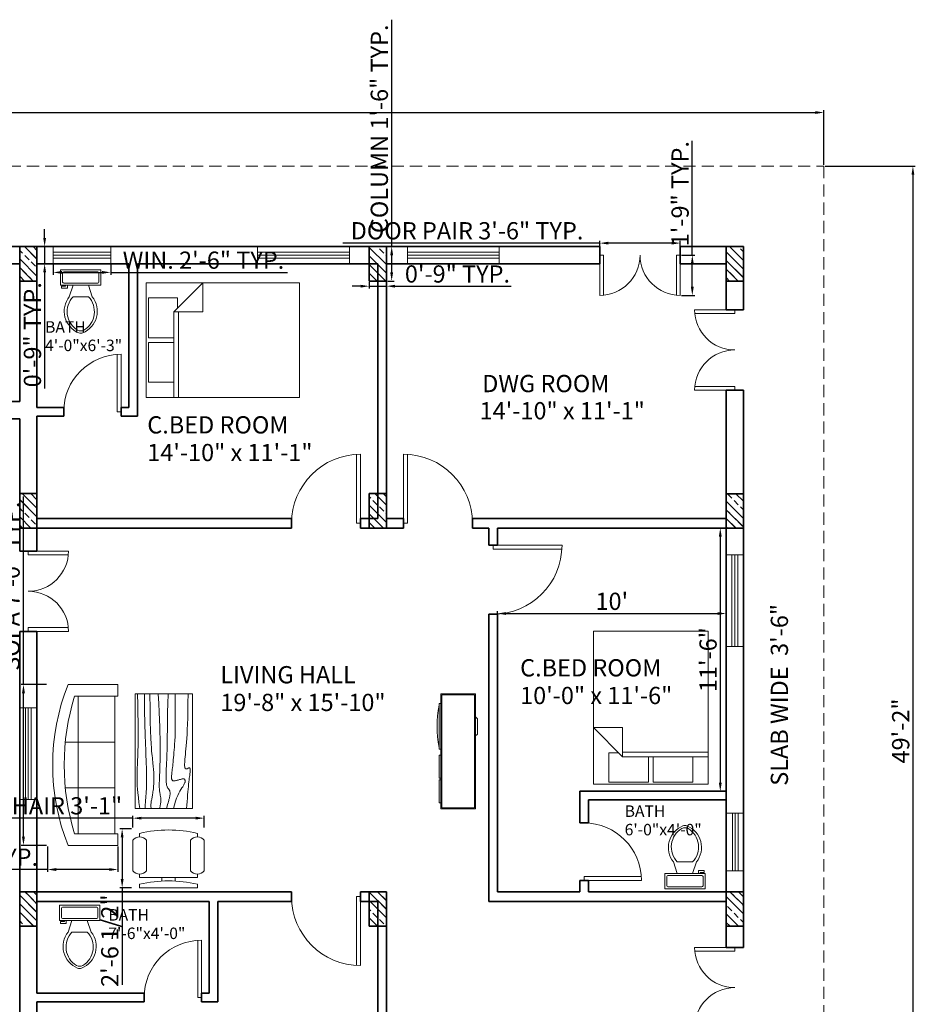
# Model space of a CAD drawing. Units: inches. Extents: x 2081 to 4786, y 1256 to 3802.
# Tile 7 of 7: x 2685 to 3153, y 1585 to 2100. Entities that reach past the tile are written whole.
import ezdxf

# ---------------------------------------------------------------- set-up
doc = ezdxf.new("R2010")
doc.units = ezdxf.units.IN
doc.linetypes.add('HIDDEN', pattern=[9.525, 6.35, -3.175])
for name, color, linetype, lineweight in [('A-ANNO-DIMS', 18, 'Continuous', 18), ('A-ANNO-TEXT', 18, 'Continuous', 18), ('A-AREA-IDEN', 18, 'Continuous', 18), ('A-COLS', 1, 'Continuous', 35), ('A-DOOR', 5, 'Continuous', 18), ('A-FLOR-FIXT', 18, 'Continuous', 18), ('A-FLOR-OVHD', 18, 'HIDDEN', 18), ('A-FURN', 5, 'Continuous', 18), ('A-GLAZ', 11, 'Continuous', 18), ('A-WALL', 7, 'Continuous', 35)]:
    doc.layers.add(name, color=color, linetype=linetype, lineweight=lineweight)
doc.styles.get("Standard").update_dxf_attribs({"font": 'arial.ttf'})
doc.dimstyles.new('ISO-25', dxfattribs={"dimtxt": 9, "dimasz": 4.5, "dimexe": 1.25, "dimexo": 0.625, "dimtad": 1, "dimdec": 0, "dimlunit": 3, "dimtxsty": 'Standard', "dimcen": 2.5, "dimadec": 0, "dimazin": 0, "dimtfac": 1, "dimtdec": 0, "dimtmove": 0, "dimatfit": 3, "dimfxl": 1, "dimarcsym": 0})
pattern_1 = [(135, (1916.44, -3174.735), (-13.47038, -13.47038), []), (135, (1916.44, -3170.245), (-13.47038, -13.47038), []), (135, (1916.44, -3165.755), (-13.47038, -13.47038), []), (135, (1916.44, -3161.265), (-13.47038, -13.47038), [])]

# ---------------------------------------------------------------- blocks, each defined once
blk = doc.blocks.new('Bed - Queen')
for p, q in [((0, -80.00003), (0, 0)), ((0, 0), (59.99999, 0)), ((59.99999, 0), (59.99999, -80.00003)), ((7.99999, -1.2), (28.79998, -1.2)), ((7.99999, -14.4), (7.99999, -1.2)), ((28.79998, -1.2), (28.79998, -14.4)), ((31.19999, -1.2), (51.99999, -1.2)), ((31.19999, -14.4), (31.19999, -1.2)), ((51.99999, -1.2), (51.99999, -16.4)), ((0, -14.4), (44.8, -14.4)), ((59.99999, -29.6), (44.8, -14.4)), ((44.8, -14.4), (44.8, -29.6)), ((44.8, -16.8), (0, -16.8)), ((51.99999, -16.4), (46.79936, -16.4)), ((44.8, -29.6), (59.99999, -29.6)), ((59.99999, -80.00003), (0, -80.00003))]:
    blk.add_line(p, q)
blk = doc.blocks.new('Sofa - Roundback 7 ft.')
for p, q in [((-12.00002, -32.4421), (-12.00003, -6.5971)), ((11.99997, -32.4421), (11.99998, -6.5971)), ((-36.000027, -34), (-36.000027, -11.4696)), ((-35.999844, -13.3819), (35.9998, -13.3819)), ((35.99998, -34), (35.99998, -11.4696)), ((-36.000027, -32.4421), (35.99998, -32.4421))]:
    blk.add_line(p, q)
for points in [[(-36.000027, -34), (-42.000027, -34), (-42.000027, -8)], [(41.99998, -8), (41.99998, -34), (35.99998, -34)]]:
    blk.add_lwpolyline(points)
for centre, radius, start, end in [((0, -114.25), 114.25, 68.43141, 111.5686), ((-0.00001, -127.1968), 121.1968, 72.72033, 107.2797)]:
    blk.add_arc(centre, radius, start, end)
blk = doc.blocks.new('Table - Rectangular Woodgrain 60 x 30 in.')
for p, q in [((0, 0), (0, -30)), ((60, 0), (0, 0)), ((60, -30), (60, 0)), ((0, -30), (60, -30))]:
    blk.add_line(p, q)
for points in [[(0, -2.4), (4.8155, -2.418), (9.0302, -2.4688), (12.709, -2.5477), (15.9167, -2.65), (18.7181, -2.7711), (21.1781, -2.9063), (23.3616, -3.0508), (25.3333, -3.2), (27.1477, -3.3495), (28.8172, -3.4958), (30.3437, -3.636), (31.7291, -3.7667), (32.9756, -3.8849), (34.0849, -3.9875), (35.059, -4.0714), (35.9, -4.1334), (36.6114, -4.1711), (37.2041, -4.1854), (37.6906, -4.1779), (38.0833, -4.15), (38.3948, -4.1034), (38.6375, -4.0396), (38.8239, -3.9602), (38.9666, -3.8667), (39.0764, -3.7608), (39.1573, -3.6448), (39.2116, -3.521), (39.2416, -3.3917), (39.2498, -3.2593), (39.2385, -3.1261), (39.21, -2.9944), (39.1666, -2.8667), (39.111, -2.7447), (39.0468, -2.6281), (38.978, -2.5163), (38.9083, -2.4083), (38.8418, -2.3035), (38.7823, -2.201), (38.7337, -2.1001), (38.7, -2), (38.6844, -1.9003), (38.6875, -1.8021), (38.7094, -1.707), (38.75, -1.6167), (38.8094, -1.5326), (38.8875, -1.4563), (38.9844, -1.3893), (39.1, -1.3333), (39.2351, -1.2896), (39.3937, -1.2583), (39.5804, -1.2396), (39.8, -1.2333), (40.057, -1.2396), (40.3562, -1.2583), (40.7023, -1.2896), (41.1, -1.3333), (41.5547, -1.3895), (42.0755, -1.4573), (42.6721, -1.5361), (43.3542, -1.625), (44.1316, -1.7233), (45.014, -1.8302), (46.0114, -1.9449), (47.1333, -2.0667), (48.3862, -2.1947), (49.7625, -2.3281), (51.2513, -2.4663), (52.8416, -2.6083), (54.5226, -2.7535), (56.2833, -2.9011), (58.1127, -3.0501), (60, -3.2)], [(0, -9.2), (6.5759, -9.0858), (11.9385, -9.0365), (16.2527, -9.0418), (19.6833, -9.0917), (22.3952, -9.1759), (24.5531, -9.2844), (26.322, -9.4069), (27.8666, -9.5333), (29.3241, -9.6553), (30.7203, -9.7719), (32.0532, -9.8837), (33.3208, -9.9917), (34.5213, -10.0965), (35.6526, -10.199), (36.7128, -10.2999), (37.7, -10.4), (38.6129, -10.4996), (39.4531, -10.5969), (40.223, -10.6895), (40.925, -10.775), (41.5613, -10.8512), (42.1344, -10.9156), (42.6465, -10.966), (43.1, -11), (43.4976, -11.0158), (43.8437, -11.0136), (44.143, -10.9942), (44.4, -10.9583), (44.6195, -10.9069), (44.8062, -10.8406), (44.9648, -10.7603), (45.1, -10.6667), (45.2155, -10.5598), (45.3114, -10.4365), (45.3871, -10.2929), (45.4416, -10.125), (45.4743, -9.929), (45.4844, -9.7011), (45.4709, -9.4371), (45.4333, -9.1333), (45.3716, -8.7883), (45.2896, -8.4104), (45.1919, -8.0107), (45.0833, -7.6), (44.9685, -7.1893), (44.8521, -6.7896), (44.7388, -6.4117), (44.6333, -6.0667), (44.54, -5.7628), (44.4614, -5.4979), (44.4001, -5.2675), (44.3583, -5.0667), (44.3384, -4.8909), (44.3427, -4.7354), (44.3736, -4.5956), (44.4333, -4.4667), (44.5236, -4.3453), (44.6427, -4.2333), (44.7884, -4.1339), (44.9583, -4.05), (45.1501, -3.9849), (45.3614, -3.9417), (45.59, -3.9234), (45.8333, -3.9333), (46.0915, -3.9749), (46.3734, -4.0531), (46.6906, -4.1736), (47.0542, -4.3417), (47.4756, -4.5629), (47.9661, -4.8427), (48.5372, -5.1866), (49.2, -5.6), (49.9676, -6.0844), (50.8594, -6.625), (51.8965, -7.2031), (53.1, -7.8), (54.491, -8.3969), (56.0906, -8.975), (57.9199, -9.5156), (60, -10)], [(0, -12.8), (5.1847, -12.9322), (9.6213, -13.0323), (13.3963, -13.1059), (16.5958, -13.1583), (19.3063, -13.1952), (21.614, -13.2219), (23.6054, -13.2439), (25.3666, -13.2667), (26.9728, -13.2947), (28.4531, -13.3281), (29.8256, -13.3663), (31.1083, -13.4083), (32.3191, -13.4535), (33.476, -13.501), (34.597, -13.5501), (35.7, -13.6), (36.7984, -13.6497), (37.8875, -13.6979), (38.9578, -13.743), (40, -13.7833), (41.0047, -13.8174), (41.9625, -13.8438), (42.864, -13.8607), (43.7, -13.8667), (44.4631, -13.8604), (45.1552, -13.8417), (45.7801, -13.8104), (46.3416, -13.7667), (46.8439, -13.7104), (47.2906, -13.6417), (47.6858, -13.5604), (48.0333, -13.4667), (48.3375, -13.3608), (48.6042, -13.2448), (48.8396, -13.121), (49.05, -12.9917), (49.2417, -12.8593), (49.4208, -12.7261), (49.5937, -12.5944), (49.7667, -12.4667), (49.9452, -12.3451), (50.1323, -12.2313), (50.3303, -12.1268), (50.5416, -12.0333), (50.7686, -11.9524), (51.0135, -11.8854), (51.2788, -11.8341), (51.5666, -11.8), (51.8785, -11.7843), (52.2116, -11.7865), (52.562, -11.8059), (52.926, -11.8417), (53.2998, -11.8931), (53.6795, -11.9594), (54.0614, -12.0397), (54.4416, -12.1333), (54.8223, -12.2401), (55.2293, -12.3625), (55.6942, -12.5037), (56.2489, -12.6667), (56.9251, -12.8547), (57.7545, -13.0708), (58.7689, -13.3182), (60, -13.6)], [(0, -18), (5.124, -17.7273), (9.6609, -17.5057), (13.6705, -17.3303), (17.2125, -17.1958), (20.3467, -17.0973), (23.1328, -17.0297), (25.6307, -16.9878), (27.9, -16.9667), (29.9928, -16.9617), (31.9302, -16.9703), (33.7254, -16.9907), (35.3917, -17.0208), (36.9423, -17.0588), (38.3906, -17.1026), (39.7499, -17.1503), (41.0333, -17.2), (42.2519, -17.2496), (43.4073, -17.2969), (44.4986, -17.3395), (45.525, -17.375), (46.4858, -17.4012), (47.3802, -17.4156), (48.2074, -17.416), (48.9667, -17.4), (49.6583, -17.3662), (50.2872, -17.3167), (50.8595, -17.2547), (51.3812, -17.1833), (51.8584, -17.1057), (52.2971, -17.025), (52.7034, -16.9443), (53.0833, -16.8667), (53.443, -16.7951), (53.789, -16.7313), (54.128, -16.6768), (54.4666, -16.6334), (54.8115, -16.6024), (55.1693, -16.5854), (55.5465, -16.5841), (55.95, -16.6), (56.3828, -16.6337), (56.8346, -16.6823), (57.2915, -16.7418), (57.7396, -16.8084), (58.165, -16.878), (58.5539, -16.9469), (58.8924, -17.0111), (59.1666, -17.0667), (59.3679, -17.1107), (59.5078, -17.1438), (59.6032, -17.1675), (59.6708, -17.1833), (59.7275, -17.193), (59.7901, -17.1979), (59.8753, -17.1998), (60, -17.2)], [(0, -22.4), (8.0098, -22.2501), (14.4094, -22.1011), (19.4168, -21.9535), (23.25, -21.8083), (26.1269, -21.6663), (28.2656, -21.5281), (29.884, -21.3947), (31.2, -21.2667), (32.3967, -21.1448), (33.5172, -21.0292), (34.5697, -20.9198), (35.5625, -20.8167), (36.5037, -20.7198), (37.4015, -20.6292), (38.2642, -20.5448), (39.1, -20.4667), (39.9164, -20.3951), (40.7187, -20.3313), (41.5117, -20.2768), (42.3, -20.2333), (43.0883, -20.2024), (43.8812, -20.1854), (44.6836, -20.1841), (45.5, -20.2), (46.3328, -20.234), (47.1747, -20.2844), (48.0163, -20.3488), (48.8479, -20.425), (49.66, -20.5106), (50.4429, -20.6031), (51.1872, -20.7004), (51.8833, -20.8), (52.5246, -20.8999), (53.1166, -20.9995), (53.6681, -21.0983), (54.1875, -21.1958), (54.6834, -21.2919), (55.1646, -21.3859), (55.6394, -21.4777), (56.1167, -21.5667), (56.6028, -21.6515), (57.0961, -21.7266), (57.5929, -21.7852), (58.0896, -21.8208), (58.5823, -21.8268), (59.0674, -21.7964), (59.5412, -21.723), (60, -21.6)], [(0, -25.2), (8.6355, -25.0504), (15.7026, -24.9031), (21.4049, -24.7606), (25.9458, -24.625), (29.529, -24.4988), (32.3578, -24.3844), (34.6359, -24.284), (36.5667, -24.2), (38.3213, -24.1341), (39.9417, -24.0854), (41.437, -24.0523), (42.8167, -24.0333), (44.0901, -24.0268), (45.2667, -24.0313), (46.3557, -24.0451), (47.3667, -24.0667), (48.309, -24.0947), (49.1928, -24.1287), (50.0284, -24.168), (50.826, -24.2125), (51.5959, -24.2617), (52.3483, -24.3151), (53.0935, -24.3725), (53.8417, -24.4334), (54.6009, -24.497), (55.3699, -24.561), (56.1454, -24.6226), (56.9239, -24.6792), (57.7021, -24.7279), (58.4764, -24.7662), (59.2435, -24.7911), (60, -24.8)], [(0, -28.8), (5.6867, -28.6681), (10.45, -28.5698), (14.407, -28.5012), (17.675, -28.4584), (20.3711, -28.4374), (22.6125, -28.4344), (24.5164, -28.4455), (26.2, -28.4667), (27.762, -28.4947), (29.2276, -28.5281), (30.6033, -28.5663), (31.8958, -28.6084), (33.1118, -28.6535), (34.2578, -28.7011), (35.3405, -28.7501), (36.3666, -28.8), (37.3443, -28.8497), (38.288, -28.8974), (39.2137, -28.9412), (40.1375, -28.9792), (41.0753, -29.0093), (42.0432, -29.0297), (43.0572, -29.0384), (44.1333, -29.0333), (45.2936, -29.0114), (46.5843, -28.9641), (48.0579, -28.8816), (49.7666, -28.7542), (51.7629, -28.5721), (54.0989, -28.3255), (56.8272, -28.0048), (60, -27.6)]]:
    blk.add_lwpolyline(points)
blk = doc.blocks.new('Entertainment Center')
for p, q in [((-4, 0), (-5, -1)), ((4, 0), (-4, 0)), ((5, -1), (4, 0)), ((-17, -19), (-17, -1)), ((-17, -1), (43, -1)), ((-16.5, -18.5), (-16.5, -1.5)), ((-16.5, -1.5), (42.5, -1.5)), ((42.5, -1.5), (42.5, -18.5)), ((43, -1), (43, -19)), ((43, -19), (-17, -19)), ((42.5, -18.5), (-16.5, -18.5)), ((-12, -20), (-12, -19)), ((12, -20), (-12, -20)), ((12, -19), (12, -20)), ((15, -20), (15, -19)), ((27, -20), (15, -20)), ((27, -19), (27, -20)), ((28, -20), (28, -19)), ((40, -20), (28, -20)), ((40, -19), (40, -20))]:
    blk.add_line(p, q)
blk.add_arc((0, 40), 61, 259.6111, 280.3889)
blk = doc.blocks.new('Chair - Desk')
for p, q in [((-8.5, 0), (-8.5, -1)), ((-8.5, 0), (8.5, 0)), ((8.5, 0), (8.5, -1)), ((-2, -3), (-2, -1.9355)), ((2, -1.9576), (2, -3)), ((-10.5, -5), (-10.5, -14)), ((-8.5, -3), (-8.5, -4)), ((-8.5, -3), (8.5, -3)), ((-6.5, -14), (-6.5, -5)), ((6.5, -5), (6.5, -14)), ((8.5, -3), (8.5, -4)), ((10.5, -14), (10.5, -5)), ((-8.5, -15), (-8.5, -16)), ((8.5, -15), (8.5, -16))]:
    blk.add_line(p, q)
for centre, radius, start, end in [((0, 34.625), 36.625, 256.5803, 283.4197), ((-8.5, -6.5), 2.5, 36.8699, 143.1301), ((8.5, -6.5), 2.5, 36.8699, 143.1301), ((-8.5, -12.5), 2.5, 216.8699, 323.1301), ((8.5, -12.5), 2.5, 216.8699, 323.1301), ((0, 19.625), 36.625, 256.5803, 283.4197)]:
    blk.add_arc(centre, radius, start, end)
blk = doc.blocks.new('Toilet - top')
for p, q in [((9.5, -6), (9.5, -2)), ((-10, -8.5), (-8, -8.5)), ((-10, -9.5), (-10, -8.5)), ((-7, -9.5), (-10, -9.5)), ((-8, -8.5), (-8, -8)), ((-7, -8), (-7, -9.5)), ((-4, -8), (-6, -14)), ((4, -8), (6, -14)), ((4, -14), (-4, -14))]:
    blk.add_line(p, q)
blk.add_lwpolyline([(10.5, -8), (10.5, 0), (-10.5, 0), (-10.5, -8)], close=True)
for points in [[(-9.5, -2), (-9.5, -6)], [(8.5, -1), (-8.5, -1)], [(-8.5, -7), (8.5, -7)]]:
    blk.add_lwpolyline(points)
for centre, radius, start, end in [((-8.62, -1.88), 0.884, 81.8699, 188.1301), ((8.62, -1.88), 0.884, 351.8699, 98.1301), ((-8.62, -6.12), 0.884, 171.8699, 278.1301), ((8.62, -6.12), 0.884, 261.8699, 8.1301), ((3.52, -21.58), 12.17, 141.4691, 247.9714), ((4.2, -21.82), 11.33, 136.3677, 238.9468), ((-3.52, -21.58), 12.17, 292.0284, 38.5307), ((-4.2, -21.82), 11.33, 301.053, 43.6321), ((0, -27.88), 4, 245.7318, 294.2682), ((0, -29), 4, 254.8605, 285.1395)]:
    blk.add_arc(centre, radius, start, end)
blk = doc.blocks.new('*D17')
at = {"layer": 'A-ANNO-DIMS', "color": 0, "lineweight": -2, "transparency": 16777216}
for p, q in [((2934.48, 1783.22), (2934.48, 1790.76)), ((3053.98, 1783.22), (3053.98, 1790.76)), ((2938.98, 1789.51), (3049.48, 1789.51))]:
    blk.add_line(p, q, dxfattribs=at)
at = {"layer": 'A-ANNO-DIMS', "color": 0, "transparency": 16777216}
for points in [[(2938.98, 1790.26), (2938.98, 1788.76), (2934.48, 1789.51)], [(3049.48, 1790.26), (3049.48, 1788.76), (3053.98, 1789.51)]]:
    blk.add_solid(points, dxfattribs=at)
at = {"layer": 'Defpoints', "color": 0, "transparency": 16777216}
for p in [(3053.98, 1789.51), (2934.48, 1782.59), (3053.98, 1782.59)]:
    blk.add_point(p, dxfattribs=at)
at = {"layer": 'A-ANNO-DIMS', "color": 0, "transparency": 16777216, "insert": (2994.23, 1794.73), "char_height": 9, "attachment_point": 5}
blk.add_mtext("10'", dxfattribs=at)
blk = doc.blocks.new('*D18')
at = {"layer": 'A-ANNO-DIMS', "color": 0, "lineweight": -2, "transparency": 16777216}
for p, q in [((2975.34, 1834.17), (3052.15, 1834.17)), ((3050.9, 1829.67), (3050.9, 1701.17)), ((2978.11, 1696.67), (3052.15, 1696.67))]:
    blk.add_line(p, q, dxfattribs=at)
at = {"layer": 'A-ANNO-DIMS', "color": 0, "transparency": 16777216}
for points in [[(3050.15, 1829.67), (3051.65, 1829.67), (3050.9, 1834.17)], [(3050.15, 1701.17), (3051.65, 1701.17), (3050.9, 1696.67)]]:
    blk.add_solid(points, dxfattribs=at)
at = {"layer": 'Defpoints', "color": 0, "transparency": 16777216}
for p in [(2974.71, 1834.17), (2977.48, 1696.67), (3050.9, 1696.67)]:
    blk.add_point(p, dxfattribs=at)
at = {"layer": 'A-ANNO-DIMS', "color": 0, "transparency": 16777216, "insert": (3045.68, 1765.42), "char_height": 9, "attachment_point": 5, "rotation": 90}
blk.add_mtext('11\'-6"', dxfattribs=at)
blk = doc.blocks.new('*D23')
at = {"layer": 'A-ANNO-DIMS', "color": 0, "lineweight": -2, "transparency": 16777216}
for p, q in [((2202.98, 2023.8), (2202.98, 2052.41)), ((3104.98, 2023.8), (3104.98, 2052.41)), ((2207.48, 2051.16), (3100.48, 2051.16))]:
    blk.add_line(p, q, dxfattribs=at)
at = {"layer": 'A-ANNO-DIMS', "color": 0, "transparency": 16777216}
for points in [[(2207.48, 2051.91), (2207.48, 2050.41), (2202.98, 2051.16)], [(3100.48, 2051.91), (3100.48, 2050.41), (3104.98, 2051.16)]]:
    blk.add_solid(points, dxfattribs=at)
at = {"layer": 'Defpoints', "color": 0, "transparency": 16777216}
for p in [(3104.98, 2051.16), (2202.98, 2023.17), (3104.98, 2023.17)]:
    blk.add_point(p, dxfattribs=at)
at = {"layer": 'A-ANNO-DIMS', "color": 0, "transparency": 16777216, "insert": (2653.98, 2056.38), "char_height": 9, "attachment_point": 5}
blk.add_mtext('75\'-2"', dxfattribs=at)
blk = doc.blocks.new('*D24')
at = {"layer": 'A-ANNO-DIMS', "color": 0, "lineweight": -2, "transparency": 16777216}
for p, q in [((3105.61, 2023.17), (3152.75, 2023.17)), ((3151.5, 2018.67), (3151.5, 1437.67)), ((3105.61, 1433.17), (3152.75, 1433.17))]:
    blk.add_line(p, q, dxfattribs=at)
at = {"layer": 'A-ANNO-DIMS', "color": 0, "transparency": 16777216}
for points in [[(3150.75, 2018.67), (3152.25, 2018.67), (3151.5, 2023.17)], [(3150.75, 1437.67), (3152.25, 1437.67), (3151.5, 1433.17)]]:
    blk.add_solid(points, dxfattribs=at)
at = {"layer": 'Defpoints', "color": 0, "transparency": 16777216}
for p in [(3104.98, 2023.17), (3104.98, 1433.17), (3151.5, 1433.17)]:
    blk.add_point(p, dxfattribs=at)
at = {"layer": 'A-ANNO-DIMS', "color": 0, "transparency": 16777216, "insert": (3146.28, 1728.17), "char_height": 9, "attachment_point": 5, "rotation": 90}
blk.add_mtext('49\'-2"', dxfattribs=at)
blk = doc.blocks.new('DOOR-PAIR-42IN')
for p, q in [((0, 42), (21, 42)), ((21, 42), (21, 40)), ((0, 40), (21, 40)), ((0, 2), (21, 2)), ((21, 0), (21, 2)), ((0, 0), (21, 0))]:
    blk.add_line(p, q)
for centre, start, end in [((21, 42), 180, 270), ((21, 0), 90, 180)]:
    blk.add_arc(centre, 21, start, end)
blk = doc.blocks.new('DOOR-SINGLE-36IN')
for p, q in [((34, 36), (34, 0)), ((36, 36), (36, 0)), ((36, 0), (34, 0))]:
    blk.add_line(p, q)
blk.add_arc((36, 0), 36, 90, 180)
blk = doc.blocks.new('DOOR-SINGLE-30IN')
for p, q in [((0, 30), (30, 30)), ((0, 28), (30, 28)), ((30, 30), (30, 28))]:
    blk.add_line(p, q)
blk.add_arc((30, 30), 30, 180, 270)
blk = doc.blocks.new('WINDOW-48IN')
for p, q in [((0, 0), (0, 9)), ((0, 9), (4, 9)), ((48, 6), (0, 6)), ((4, 9), (48, 9)), ((48, 0), (48, 9)), ((48, 4.5), (0, 4.5)), ((48, 3), (0, 3)), ((48, 0), (0, 0))]:
    blk.add_line(p, q)
blk = doc.blocks.new('WINDOW-30IN')
for p, q in [((0, 0), (0, 30)), ((0, 30), (9, 30)), ((3, 0), (3, 30)), ((4.5, 0), (4.5, 30)), ((6, 0), (6, 30)), ((9, 30), (9, 0)), ((9, 0), (0, 0))]:
    blk.add_line(p, q)
blk = doc.blocks.new('COLUMN-9X18IN')
h = blk.add_hatch()
h.set_pattern_fill('ANSI34', color=256, angle=90)
h.set_pattern_definition(pattern_1)
h.paths.add_polyline_path([(9, 18), (0, 18), (0, 0), (9, 0)])
h = blk.add_hatch()
h.set_pattern_fill('ANSI34', color=256, angle=90)
h.set_pattern_definition(pattern_1)
h.paths.add_polyline_path([(9, 18), (0, 18), (0, 0), (9, 0)])
h = blk.add_hatch()
h.set_pattern_fill('ANSI34', color=256, angle=90)
h.set_pattern_definition(pattern_1)
h.paths.add_polyline_path([(9, 18), (0, 18), (0, 0), (9, 0)])
h = blk.add_hatch()
h.set_pattern_fill('ANSI33', color=256, angle=90)
h.set_pattern_definition([(135, (1916.44, -3174.7355), (-4.490128, -4.490128), []), (135, (1916.44, -3170.2454), (-4.490128, -4.490128), [3.175, -1.5875])])
h.paths.add_polyline_path([(0, 0), (9, 0), (9, 18), (0, 18)])
for p, q in [((0, 0), (0, 18)), ((0, 18), (9, 18)), ((9, 18), (9, 0)), ((9, 0), (0, 0))]:
    blk.add_line(p, q)
blk = doc.blocks.new('*D33')
at = {"layer": 'A-ANNO-DIMS', "color": 0, "lineweight": -2, "transparency": 16777216}
for p, q in [((2879.27, 1981.17), (2879.27, 2099.66)), ((2877.19, 1981.17), (2880.52, 1981.17)), ((2879.27, 1967.67), (2879.27, 1976.67)), ((2877.19, 1963.17), (2880.52, 1963.17))]:
    blk.add_line(p, q, dxfattribs=at)
at = {"layer": 'A-ANNO-DIMS', "color": 0, "transparency": 16777216}
for points in [[(2878.52, 1976.67), (2880.02, 1976.67), (2879.27, 1981.17)], [(2878.52, 1967.67), (2880.02, 1967.67), (2879.27, 1963.17)]]:
    blk.add_solid(points, dxfattribs=at)
at = {"layer": 'Defpoints', "color": 0, "transparency": 16777216}
for p in [(2876.57, 1981.17), (2879.27, 1981.17), (2876.57, 1963.17)]:
    blk.add_point(p, dxfattribs=at)
at = {"layer": 'A-ANNO-DIMS', "color": 0, "transparency": 16777216, "insert": (2873.99, 2042.66), "char_height": 9, "attachment_point": 5, "rotation": 90}
blk.add_mtext('COLUMN 1\'-6" TYP.', dxfattribs=at)
blk = doc.blocks.new('*D34')
at = {"layer": 'A-ANNO-DIMS', "color": 0, "lineweight": -2, "transparency": 16777216}
for p, q in [((2863.07, 1960.47), (2858.57, 1960.47)), ((2867.57, 1962.55), (2867.57, 1959.22)), ((2867.57, 1960.47), (2876.57, 1960.47)), ((2876.57, 1962.55), (2876.57, 1959.22)), ((2881.07, 1960.47), (2941.68, 1960.47))]:
    blk.add_line(p, q, dxfattribs=at)
at = {"layer": 'A-ANNO-DIMS', "color": 0, "transparency": 16777216}
for points in [[(2863.07, 1961.22), (2863.07, 1959.72), (2867.57, 1960.47)], [(2881.07, 1961.22), (2881.07, 1959.72), (2876.57, 1960.47)]]:
    blk.add_solid(points, dxfattribs=at)
at = {"layer": 'Defpoints', "color": 0, "transparency": 16777216}
for p in [(2867.57, 1963.17), (2876.57, 1963.17), (2876.57, 1960.47)]:
    blk.add_point(p, dxfattribs=at)
at = {"layer": 'A-ANNO-DIMS', "color": 0, "transparency": 16777216, "insert": (2913.62, 1965.69), "char_height": 9, "attachment_point": 5}
blk.add_mtext('0\'-9" TYP.', dxfattribs=at)
blk = doc.blocks.new('*D43')
at = {"layer": 'A-ANNO-DIMS', "color": 0, "lineweight": -2, "transparency": 16777216}
for p, q in [((2987.98, 1982.97), (2853.77, 1982.97)), ((2987.98, 1977.3), (2987.98, 1984.22)), ((3025.48, 1982.97), (2992.48, 1982.97)), ((3029.98, 1977.3), (3029.98, 1984.22))]:
    blk.add_line(p, q, dxfattribs=at)
at = {"layer": 'A-ANNO-DIMS', "color": 0, "transparency": 16777216}
for points in [[(2992.48, 1983.72), (2992.48, 1982.22), (2987.98, 1982.97)], [(3025.48, 1983.72), (3025.48, 1982.22), (3029.98, 1982.97)]]:
    blk.add_solid(points, dxfattribs=at)
at = {"layer": 'Defpoints', "color": 0, "transparency": 16777216}
for p in [(2987.98, 1982.97), (2987.98, 1976.67), (3029.98, 1976.67)]:
    blk.add_point(p, dxfattribs=at)
at = {"layer": 'A-ANNO-DIMS', "color": 0, "transparency": 16777216, "insert": (2918.63, 1988.26), "char_height": 9, "attachment_point": 5}
blk.add_mtext('DOOR PAIR 3\'-6" TYP.', dxfattribs=at)
blk = doc.blocks.new('*D44')
at = {"layer": 'A-ANNO-DIMS', "color": 0, "lineweight": -2, "transparency": 16777216}
for p, q in [((3036.28, 1976.67), (3036.28, 2036.44)), ((3030.61, 1976.67), (3037.53, 1976.67)), ((3036.28, 1960.17), (3036.28, 1972.17)), ((3030.61, 1955.67), (3037.53, 1955.67))]:
    blk.add_line(p, q, dxfattribs=at)
at = {"layer": 'A-ANNO-DIMS', "color": 0, "transparency": 16777216}
for points in [[(3035.53, 1972.17), (3037.03, 1972.17), (3036.28, 1976.67)], [(3035.53, 1960.17), (3037.03, 1960.17), (3036.28, 1955.67)]]:
    blk.add_solid(points, dxfattribs=at)
at = {"layer": 'Defpoints', "color": 0, "transparency": 16777216}
for p in [(3029.98, 1976.67), (3036.28, 1976.67), (3029.98, 1955.67)]:
    blk.add_point(p, dxfattribs=at)
at = {"layer": 'A-ANNO-DIMS', "color": 0, "transparency": 16777216, "insert": (3031.06, 2008.8), "char_height": 9, "attachment_point": 5, "rotation": 90}
blk.add_mtext('1\'-9" TYP.', dxfattribs=at)
blk = doc.blocks.new('*D47')
at = {"layer": 'A-ANNO-DIMS', "color": 0, "lineweight": -2, "transparency": 16777216}
for p, q in [((2702.52, 1971.55), (2702.52, 1966.42)), ((2732.52, 1971.55), (2732.52, 1966.42)), ((2707.02, 1967.67), (2728.02, 1967.67)), ((2732.52, 1967.67), (2824.93, 1967.67))]:
    blk.add_line(p, q, dxfattribs=at)
at = {"layer": 'A-ANNO-DIMS', "color": 0, "transparency": 16777216}
for points in [[(2707.02, 1968.42), (2707.02, 1966.92), (2702.52, 1967.67)], [(2728.02, 1968.42), (2728.02, 1966.92), (2732.52, 1967.67)]]:
    blk.add_solid(points, dxfattribs=at)
at = {"layer": 'Defpoints', "color": 0, "transparency": 16777216}
for p in [(2702.52, 1972.17), (2732.52, 1972.17), (2732.52, 1967.67)]:
    blk.add_point(p, dxfattribs=at)
at = {"layer": 'A-ANNO-DIMS', "color": 0, "transparency": 16777216, "insert": (2780.98, 1972.89), "char_height": 9, "attachment_point": 5}
blk.add_mtext('WIN. 2\'-6" TYP.', dxfattribs=at)
blk = doc.blocks.new('*D48')
at = {"layer": 'A-ANNO-DIMS', "color": 0, "lineweight": -2, "transparency": 16777216}
for p, q in [((2698.02, 1985.67), (2698.02, 1990.17)), ((2701.9, 1981.17), (2696.77, 1981.17)), ((2698.02, 1981.17), (2698.02, 1972.17)), ((2701.9, 1972.17), (2696.77, 1972.17)), ((2698.02, 1967.67), (2698.02, 1907.06))]:
    blk.add_line(p, q, dxfattribs=at)
at = {"layer": 'A-ANNO-DIMS', "color": 0, "transparency": 16777216}
for points in [[(2697.27, 1985.67), (2698.77, 1985.67), (2698.02, 1981.17)], [(2697.27, 1967.67), (2698.77, 1967.67), (2698.02, 1972.17)]]:
    blk.add_solid(points, dxfattribs=at)
at = {"layer": 'Defpoints', "color": 0, "transparency": 16777216}
for p in [(2702.52, 1981.17), (2698.02, 1972.17), (2702.52, 1972.17)]:
    blk.add_point(p, dxfattribs=at)
at = {"layer": 'A-ANNO-DIMS', "color": 0, "transparency": 16777216, "insert": (2692.8, 1935.12), "char_height": 9, "attachment_point": 5, "rotation": 90}
blk.add_mtext('0\'-9" TYP.', dxfattribs=at)
blk = doc.blocks.new('*D51')
at = {"layer": 'A-ANNO-DIMS', "color": 0, "lineweight": -2, "transparency": 16777216}
for p, q in [((2744.09, 1682.64), (2671.91, 1682.64)), ((2744.09, 1677.68), (2744.09, 1683.89)), ((2776.84, 1682.64), (2748.59, 1682.64)), ((2781.34, 1677.68), (2781.34, 1683.89))]:
    blk.add_line(p, q, dxfattribs=at)
at = {"layer": 'A-ANNO-DIMS', "color": 0, "transparency": 16777216}
for points in [[(2748.59, 1683.39), (2748.59, 1681.89), (2744.09, 1682.64)], [(2776.84, 1683.39), (2776.84, 1681.89), (2781.34, 1682.64)]]:
    blk.add_solid(points, dxfattribs=at)
at = {"layer": 'Defpoints', "color": 0, "transparency": 16777216}
for p in [(2744.09, 1682.64), (2744.09, 1677.06), (2781.34, 1677.06)]:
    blk.add_point(p, dxfattribs=at)
at = {"layer": 'A-ANNO-DIMS', "color": 0, "transparency": 16777216, "insert": (2705.75, 1687.93), "char_height": 9, "attachment_point": 5}
blk.add_mtext('CHAIR 3\'-1"', dxfattribs=at)
blk = doc.blocks.new('*D52')
at = {"layer": 'A-ANNO-DIMS', "color": 0, "lineweight": -2, "transparency": 16777216}
for p, q in [((2743.46, 1677.06), (2737.25, 1677.06)), ((2738.5, 1672.56), (2738.5, 1650.81)), ((2743.46, 1646.31), (2737.25, 1646.31)), ((2738.5, 1646.31), (2738.5, 1595.52))]:
    blk.add_line(p, q, dxfattribs=at)
at = {"layer": 'A-ANNO-DIMS', "color": 0, "transparency": 16777216}
for points in [[(2737.75, 1672.56), (2739.25, 1672.56), (2738.5, 1677.06)], [(2737.75, 1650.81), (2739.25, 1650.81), (2738.5, 1646.31)]]:
    blk.add_solid(points, dxfattribs=at)
at = {"layer": 'Defpoints', "color": 0, "transparency": 16777216}
for p in [(2744.09, 1677.06), (2738.5, 1646.31), (2744.09, 1646.31)]:
    blk.add_point(p, dxfattribs=at)
at = {"layer": 'A-ANNO-DIMS', "color": 0, "transparency": 16777216, "insert": (2733.22, 1618.66), "char_height": 9, "attachment_point": 5, "rotation": 90}
blk.add_mtext('2\'-6 1/2"', dxfattribs=at)
blk = doc.blocks.new('*D55')
at = {"layer": 'A-ANNO-DIMS', "color": 0, "lineweight": -2, "transparency": 16777216}
for p, q in [((2686.95, 1752.41), (2686.95, 1850.7)), ((2698.93, 1752.41), (2685.7, 1752.41)), ((2686.95, 1672.91), (2686.95, 1747.91)), ((2698.93, 1668.41), (2685.7, 1668.41))]:
    blk.add_line(p, q, dxfattribs=at)
at = {"layer": 'A-ANNO-DIMS', "color": 0, "transparency": 16777216}
for points in [[(2686.2, 1747.91), (2687.7, 1747.91), (2686.95, 1752.41)], [(2686.2, 1672.91), (2687.7, 1672.91), (2686.95, 1668.41)]]:
    blk.add_solid(points, dxfattribs=at)
at = {"layer": 'Defpoints', "color": 0, "transparency": 16777216}
for p in [(2686.95, 1752.41), (2699.55, 1752.41), (2699.55, 1668.41)]:
    blk.add_point(p, dxfattribs=at)
at = {"layer": 'A-ANNO-DIMS', "color": 0, "transparency": 16777216, "insert": (2681.67, 1803.8), "char_height": 9, "attachment_point": 5, "rotation": 90}
blk.add_mtext('SOFA 7\'-0" TYP.', dxfattribs=at)
blk = doc.blocks.new('*D56')
at = {"layer": 'A-ANNO-DIMS', "color": 0, "lineweight": -2, "transparency": 16777216}
for p, q in [((2699.55, 1667.78), (2699.55, 1654.56)), ((2736.22, 1667.78), (2736.22, 1654.56)), ((2699.55, 1655.81), (2617.98, 1655.81)), ((2731.72, 1655.81), (2704.05, 1655.81))]:
    blk.add_line(p, q, dxfattribs=at)
at = {"layer": 'A-ANNO-DIMS', "color": 0, "transparency": 16777216}
for points in [[(2704.05, 1656.56), (2704.05, 1655.06), (2699.55, 1655.81)], [(2731.72, 1656.56), (2731.72, 1655.06), (2736.22, 1655.81)]]:
    blk.add_solid(points, dxfattribs=at)
at = {"layer": 'Defpoints', "color": 0, "transparency": 16777216}
for p in [(2699.55, 1668.41), (2736.22, 1668.41), (2699.55, 1655.81)]:
    blk.add_point(p, dxfattribs=at)
at = {"layer": 'A-ANNO-DIMS', "color": 0, "transparency": 16777216, "insert": (2656.52, 1661.09), "char_height": 9, "attachment_point": 5}
blk.add_mtext('3\'-0 1/2" TYP.', dxfattribs=at)

msp = doc.modelspace()

# ---------------------------------------------------------------- linework, layer by layer
at = {"layer": 'A-FLOR-OVHD'}
for p, q in [((2202.98, 2023.17), (3062.98, 2023.17)), ((3062.98, 2023.17), (3104.98, 2023.17)), ((3104.98, 2023.17), (3104.98, 1433.17))]:
    msp.add_line(p, q, dxfattribs=at)
at = {"layer": 'A-WALL'}
for p, q in [((2579.98, 1981.17), (2987.98, 1981.17)), ((2987.98, 1981.17), (2987.98, 1972.17)), ((3029.98, 1981.17), (3062.98, 1981.17)), ((3029.98, 1981.17), (3029.98, 1972.17)), ((3062.98, 1981.17), (3062.98, 1948.17)), ((2600.98, 1972.17), (2684.98, 1972.17)), ((2684.98, 1900.17), (2684.98, 1972.17)), ((2693.98, 1897.17), (2693.98, 1972.17)), ((2693.98, 1972.17), (2741.98, 1972.17)), ((2741.98, 1897.17), (2741.98, 1972.17)), ((2746.48, 1892.67), (2746.48, 1972.17)), ((2746.48, 1972.17), (2871.98, 1972.17)), ((2871.98, 1839.17), (2871.98, 1972.17)), ((2876.48, 1839.17), (2876.48, 1972.17)), ((2876.48, 1972.17), (2987.98, 1972.17)), ((3029.98, 1972.17), (3053.98, 1972.17)), ((3053.98, 1972.17), (3053.98, 1948.17)), ((3053.98, 1948.17), (3062.98, 1948.17)), ((3053.98, 1906.17), (3062.98, 1906.17)), ((3053.98, 1906.17), (3053.98, 1839.17)), ((3062.98, 1906.17), (3062.98, 1615.17)), ((2669.98, 1900.17), (2684.98, 1900.17)), ((2693.98, 1897.17), (2707.98, 1897.17)), ((2693.98, 1892.67), (2707.98, 1892.67)), ((2693.98, 1839.17), (2693.98, 1892.67)), ((2707.98, 1892.67), (2707.98, 1897.17)), ((2737.98, 1892.67), (2737.98, 1897.17)), ((2737.98, 1897.17), (2741.98, 1897.17)), ((2737.98, 1892.67), (2746.48, 1892.67)), ((2669.98, 1891.17), (2684.98, 1891.17)), ((2684.98, 1822.17), (2684.98, 1891.17)), ((2693.98, 1839.17), (2826.98, 1839.17)), ((2826.98, 1834.17), (2826.98, 1839.17)), ((2862.98, 1834.17), (2862.98, 1839.17)), ((2862.98, 1839.17), (2871.98, 1839.17)), ((2876.48, 1839.17), (2885.48, 1839.17)), ((2885.48, 1834.17), (2885.48, 1839.17)), ((2921.48, 1834.17), (2921.48, 1839.17)), ((2921.48, 1839.17), (3053.98, 1839.17)), ((2693.98, 1834.17), (2826.98, 1834.17)), ((2693.98, 1822.17), (2693.98, 1834.17)), ((2862.98, 1834.17), (2885.48, 1834.17)), ((2921.48, 1834.17), (2929.98, 1834.17)), ((2929.98, 1825.17), (2929.98, 1834.17)), ((2934.48, 1825.17), (2934.48, 1834.17)), ((2934.48, 1834.17), (3053.98, 1834.17)), ((3053.98, 1834.17), (3053.98, 1644.17)), ((2684.98, 1822.17), (2693.98, 1822.17)), ((2929.98, 1825.17), (2934.48, 1825.17)), ((2929.98, 1639.17), (2929.98, 1789.17)), ((2929.98, 1789.17), (2934.48, 1789.17)), ((2934.48, 1644.17), (2934.48, 1789.17)), ((2684.98, 1442.17), (2684.98, 1780.17)), ((2684.98, 1780.17), (2693.98, 1780.17)), ((2693.98, 1644.17), (2693.98, 1780.17)), ((2977.48, 1696.67), (2977.48, 1680.17)), ((2977.48, 1696.67), (3053.98, 1696.67)), ((2981.98, 1692.17), (2981.98, 1680.17)), ((2981.98, 1692.17), (3053.98, 1692.17)), ((2977.48, 1680.17), (2981.98, 1680.17)), ((2977.48, 1650.17), (2981.98, 1650.17)), ((2977.48, 1650.17), (2977.48, 1644.17)), ((2981.98, 1650.17), (2981.98, 1644.17)), ((2693.98, 1644.17), (2826.98, 1644.17)), ((2826.98, 1639.17), (2826.98, 1644.17)), ((2862.98, 1639.17), (2862.98, 1644.17)), ((2862.98, 1644.17), (2876.48, 1644.17)), ((2876.48, 1442.17), (2876.48, 1644.17)), ((2934.48, 1644.17), (2977.48, 1644.17)), ((2981.98, 1644.17), (3053.98, 1644.17)), ((2693.98, 1639.17), (2783.98, 1639.17)), ((2693.98, 1591.17), (2693.98, 1639.17)), ((2783.98, 1591.17), (2783.98, 1639.17)), ((2788.48, 1586.67), (2788.48, 1639.17)), ((2788.48, 1639.17), (2826.98, 1639.17)), ((2862.98, 1639.17), (2871.98, 1639.17)), ((2871.98, 1442.17), (2871.98, 1639.17)), ((2929.98, 1639.17), (3053.98, 1639.17)), ((3053.98, 1639.17), (3053.98, 1615.17)), ((3053.98, 1615.17), (3062.98, 1615.17)), ((2693.98, 1591.17), (2749.98, 1591.17)), ((2749.98, 1586.67), (2749.98, 1591.17)), ((2779.98, 1586.67), (2779.98, 1591.17)), ((2779.98, 1591.17), (2783.98, 1591.17)), ((2693.98, 1442.17), (2693.98, 1586.67)), ((2693.98, 1586.67), (2749.98, 1586.67)), ((2779.98, 1586.67), (2788.48, 1586.67))]:
    msp.add_line(p, q, dxfattribs=at)

# ---------------------------------------------------------------- block references
at = {"layer": 'A-COLS'}
for p in [(2685.01, 1963.17), (2867.57, 1963.17), (3053.98, 1963.17), (2685.01, 1834.17), (2867.48, 1834.17), (3053.98, 1834.1), (2684.98, 1626.17), (2867.48, 1626.17), (3053.98, 1626.17)]:
    msp.add_blockref('COLUMN-9X18IN', p, dxfattribs=at)
at = {"layer": 'A-DOOR'}
for name, p, rotation in [('DOOR-PAIR-42IN', (3029.98, 1955.67), 90.00000000000058), ('DOOR-SINGLE-30IN', (2707.98, 1924.92), 269.9999999999997), ('DOOR-PAIR-42IN', (2710.48, 1822.17), 180), ('DOOR-SINGLE-30IN', (3009.73, 1680.17), 180), ('DOOR-SINGLE-30IN', (2749.98, 1618.92), 270.0000000000001)]:
    msp.add_blockref(name, p, dxfattribs=dict(at, rotation=rotation))
for name, p in [('DOOR-PAIR-42IN', (3037.48, 1906.17)), ('DOOR-SINGLE-36IN', (2826.98, 1836.67)), ('DOOR-PAIR-42IN', (3037.48, 1573.17))]:
    msp.add_blockref(name, p, dxfattribs=at)
at = {"layer": 'A-DOOR', "extrusion": (0, 0, -1), "zscale": -1}
msp.add_blockref('DOOR-SINGLE-36IN', (-2921.48, 1836.67), dxfattribs=at)
for p, rotation in [((-2932.23, 1789.17), 90.00000000000044), ((-2826.98, 1641.67), 180)]:
    msp.add_blockref('DOOR-SINGLE-36IN', p, dxfattribs=dict(at, rotation=rotation))
at = {"layer": 'A-FLOR-FIXT'}
for p in [(2716.88, 1968.97), (2716.3, 1637.16)]:
    msp.add_blockref('Toilet - top', p, dxfattribs=at)
at = {"layer": 'A-FLOR-FIXT', "rotation": 180}
msp.add_blockref('Toilet - top', (3032.44, 1645.77), dxfattribs=at)
at = {"layer": 'A-FURN'}
for name, p, rotation in [('Bed - Queen', (2751.08, 1902.31), 90), ('Bed - Queen', (3044.63, 1700.32), 180), ('Sofa - Roundback 7 ft.', (2702.22, 1710.41), 89.99999999999999), ('Table - Rectangular Woodgrain 60 x 30 in.', (2775.3, 1747.6), 270), ('Entertainment Center', (2924.02, 1730.59), 270)]:
    msp.add_blockref(name, p, dxfattribs=dict(at, rotation=rotation))
at = {"layer": 'A-FURN', "xscale": 1.773670891908859, "yscale": 1.773670891908859, "zscale": 1.773670891908859, "rotation": 180}
msp.add_blockref('Chair - Desk', (2762.71, 1646.31), dxfattribs=at)
at = {"layer": 'A-GLAZ'}
for name, p, rotation in [('WINDOW-30IN', (2702.52, 1981.17), 270.0000000000016), ('WINDOW-48IN', (3053.98, 1820.23), 269.9999999999989), ('WINDOW-48IN', (2684.98, 1740.34), 269.9999999999987)]:
    msp.add_blockref(name, p, dxfattribs=dict(at, rotation=rotation))
for name, p in [('WINDOW-48IN', (2809.23, 1972.17)), ('WINDOW-48IN', (2887.47, 1972.17)), ('WINDOW-30IN', (3054.22, 1655.19))]:
    msp.add_blockref(name, p, dxfattribs=at)

# ---------------------------------------------------------------- texts
at = {"layer": 'A-ANNO-TEXT'}
msp.add_text('SLAB WIDE  3\'-6"', height=9, rotation=90, dxfattribs=at).set_placement((3086.26, 1699.55))
at = {"layer": 'A-AREA-IDEN'}
for s, height, p in [('BATH', 6, (2698.25, 1936.18)), ('4\'-0"x6\'-3"', 6, (2698.25, 1926.55)), ('DWG ROOM ', 9, (2926.54, 1905.12)), ('14\'-10" x 11\'-1"', 9, (2925.2, 1890.94)), ('C.BED ROOM', 9, (2751.61, 1883.55)), ('14\'-10" x 11\'-1"', 9, (2751.61, 1869.09)), ('C.BED ROOM', 9, (2946.34, 1756.66)), ('LIVING HALL', 9, (2789.77, 1753.05)), ('10\'-0" x 11\'-6"', 9, (2946.34, 1742.21)), ('19\'-8" x 15\'-10"', 9, (2789.77, 1738.59)), ('BATH', 6, (3000.95, 1683.31)), ('6\'-0"x4\'-0"', 6, (3000.95, 1673.67)), ('BATH', 6, (2731.28, 1629.14)), ('7\'-6"x4\'-0"', 6, (2731.28, 1619.5))]:
    msp.add_text(s, height=height, dxfattribs=at).set_placement(p)

# ---------------------------------------------------------------- dimensions: what is measured, and where the dimension line sits
at = {"layer": 'A-ANNO-DIMS'}
for base, p1, p2, angle, text, picture, middle in [((2879.27, 1981.17), (2876.57, 1963.17), (2876.57, 1981.17), 90, 'COLUMN <> TYP.', '*D33', (2873.99, 2042.66)), ((3036.28, 1976.67), (3029.98, 1955.67), (3029.98, 1976.67), 90, '<> TYP.', '*D44', (3031.06, 2008.8)), ((2987.98, 1982.97), (3029.98, 1976.67), (2987.98, 1976.67), 180, 'DOOR PAIR <> TYP.', '*D43', (2918.63, 1988.26)), ((2698.02, 1972.17), (2702.52, 1981.17), (2702.52, 1972.17), 270, '<> TYP.', '*D48', (2692.8, 1935.12)), ((2732.52, 1967.67), (2702.52, 1972.17), (2732.52, 1972.17), 0, 'WIN. <> TYP.', '*D47', (2780.98, 1972.89)), ((2686.95, 1752.41), (2699.55, 1668.41), (2699.55, 1752.41), 90, 'SOFA <> TYP.', '*D55', (2681.67, 1803.8)), ((2744.0897, 1682.6449), (2781.3368, 1677.0579), (2744.0897, 1677.0579), 180, 'CHAIR <>', '*D51', (2705.7488, 1687.9265)), ((2699.55, 1655.81), (2736.22, 1668.41), (2699.55, 1668.41), 180, '<> TYP.', '*D56', (2656.52, 1661.09))]:
    dim = msp.add_linear_dim(base=base, p1=p1, p2=p2, angle=angle, text=text, dimstyle='ISO-25', override={"dimdec": 1, "dimlfac": 1, "dimrnd": 0, "dimzin": 1, "dimdsep": 46, "dimlunit": 4, "dimfrac": 2}, dxfattribs=at)
    dim.commit()
    dim.dimension.update_dxf_attribs({"geometry": picture, "text_midpoint": middle})
for base, p1, p2, picture, middle in [((3104.98, 2051.16), (2202.98, 2023.17), (3104.98, 2023.17), '*D23', (2653.98, 2056.38)), ((3053.98343114, 1789.51372892), (2934.48343114, 1782.59368821), (3053.98343114, 1782.59368821), '*D17', (2994.23343114, 1794.73388581))]:
    dim = msp.add_linear_dim(base=base, p1=p1, p2=p2, dimstyle='ISO-25', override={"dimclrd": 0, "dimclre": 0, "dimclrt": 0}, dxfattribs=at)
    dim.commit()
    dim.dimension.update_dxf_attribs({"geometry": picture, "text_midpoint": middle})
for base, p1, p2, angle, override, picture, middle in [((3151.5, 1433.17), (3104.98, 2023.17), (3104.98, 1433.17), 90, {"dimclrd": 0, "dimclre": 0, "dimclrt": 0}, '*D24', (3146.28, 1728.17)), ((3050.89915939, 1696.67279746), (2974.71112297, 1834.17279746), (2977.48343114, 1696.67279746), 90, {"dimclrd": 0, "dimclre": 0, "dimclrt": 0}, '*D18', (3045.6790025, 1765.42279746)), ((2738.5026, 1646.3142), (2744.0897, 1677.0579), (2744.0897, 1646.3142), 270, {"dimdec": 1, "dimlfac": 1, "dimrnd": 0, "dimzin": 1, "dimdsep": 46, "dimlunit": 4, "dimfrac": 2}, '*D52', (2733.2242, 1618.6647))]:
    dim = msp.add_linear_dim(base=base, p1=p1, p2=p2, angle=angle, dimstyle='ISO-25', override=override, dxfattribs=at)
    dim.commit()
    dim.dimension.update_dxf_attribs({"geometry": picture, "text_midpoint": middle})
dim = msp.add_linear_dim(base=(2876.57, 1960.47), p1=(2867.57, 1963.17), p2=(2876.57, 1963.17), text='<> TYP.', dimstyle='ISO-25', override={"dimdec": 1, "dimlfac": 1, "dimrnd": 0, "dimzin": 1, "dimdsep": 46, "dimlunit": 4, "dimfrac": 2}, dxfattribs=at)
dim.commit()
dim.dimension.update_dxf_attribs({"geometry": '*D34', "text_midpoint": (2913.62, 1965.69)})

doc.saveas('drawing.dxf')
